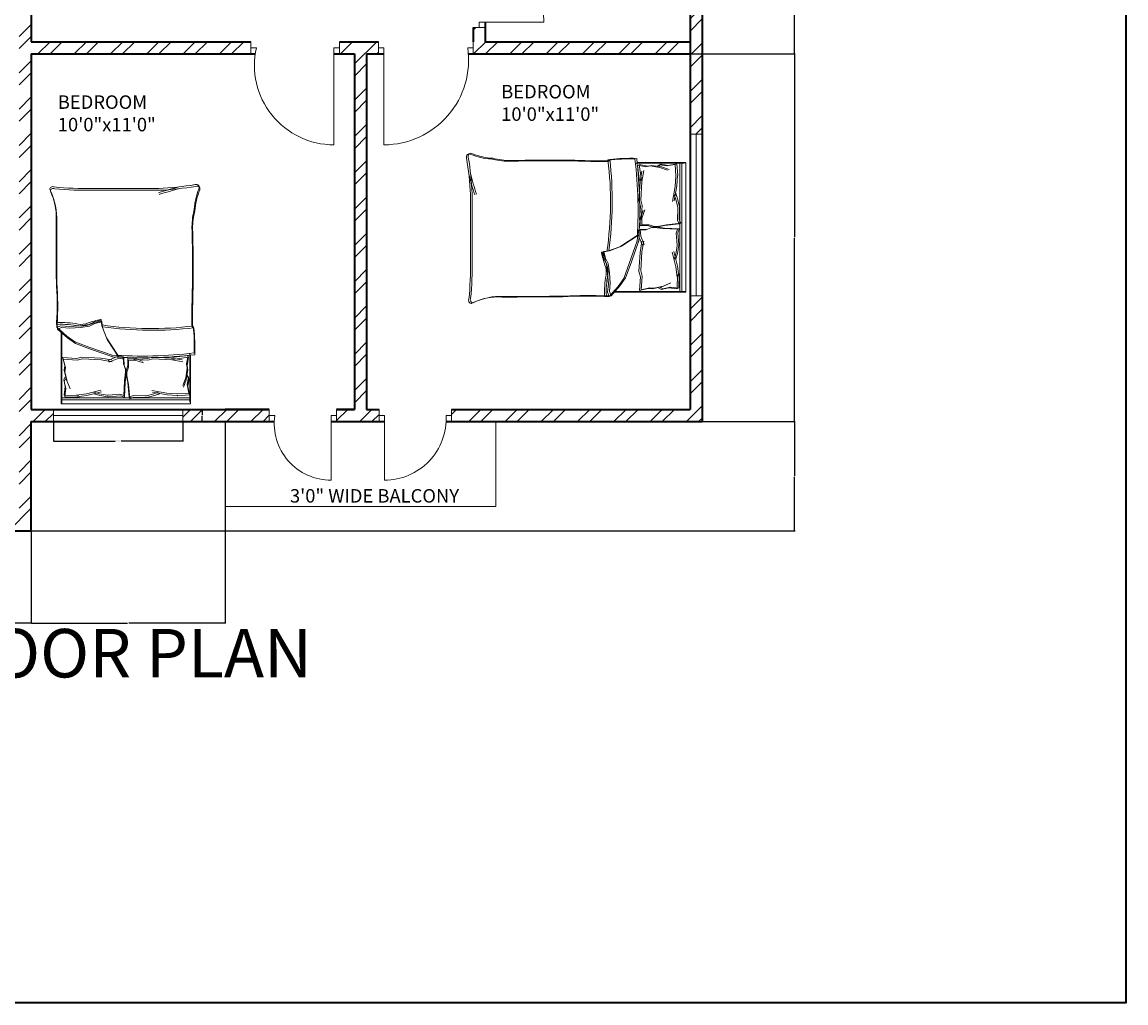
# Model space of a CAD drawing. Units: inches. Extents: x 2165 to 3042, y 1626 to 2968.
# Tile 6 of 11: x 2633 to 3042, y 1626 to 1990. Entities that reach past the tile are written whole.
import ezdxf

# ---------------------------------------------------------------- set-up
doc = ezdxf.new("R2010")
doc.units = ezdxf.units.IN
for name, color, linetype, lineweight in [('A-ANNO-DIMS', 2, 'Continuous', 18), ('A-ANNO-TEXT', 7, 'Continuous', 25), ('A-AREA-IDEN', 7, 'Continuous', 18), ('A-DOOR', 3, 'Continuous', 18), ('A-FLOR-BALC', 7, 'Continuous', 18), ('A-FURN', 8, 'Continuous', 13), ('A-GLAZ', 4, 'Continuous', 18), ('A-WALL', 7, 'Continuous', 35), ('A-WALL-PATT', 252, 'Continuous', 13)]:
    doc.layers.add(name, color=color, linetype=linetype, lineweight=lineweight)
doc.styles.get("Standard").update_dxf_attribs({"font": 'arial.ttf'})
doc.dimstyles.get("Standard").update_dxf_attribs({"dimtxt": 0.18, "dimasz": 0.18, "dimexe": 0.18, "dimexo": 0.0625, "dimgap": 0.09, "dimtad": 0, "dimtih": 1, "dimtoh": 1, "dimdec": 4, "dimzin": 0, "dimdsep": 46, "dimtxsty": 'Standard', "dimcen": 0.09, "dimadec": 0, "dimazin": 0, "dimtfac": 1, "dimtdec": 4, "dimtofl": 0, "dimtmove": 0, "dimatfit": 3, "dimfxl": 1, "dimtolj": 1, "dimtzin": 0, "dimarcsym": 0})

# ---------------------------------------------------------------- blocks, each defined once
blk = doc.blocks.new('BED-DOUBLE')
for p, q in [((0, 51.27), (0, 51.49)), ((0, 51.49), (0.64, 51.49)), ((0, 51.27), (26.61, 51.27)), ((0, 51.27), (26.61, 51.27)), ((0, 51.27), (0, 3.48)), ((0.64, 51.49), (27.25, 51.49)), ((0.64, 51.49), (27.25, 51.49)), ((1.53, 3.48), (1.53, 51.27)), ((1.53, 3.47), (1.53, 51.27)), ((2.17, 3.7), (2.17, 51.49)), ((2.17, 3.7), (2.17, 51.49)), ((2.56, 50.11), (2.46, 44.71)), ((2.56, 50.11), (2.46, 44.71)), ((2.56, 50.11), (5.77, 49.73)), ((2.56, 50.11), (5.77, 49.73)), ((3.2, 50.34), (3.1, 44.94)), ((3.2, 50.34), (3.1, 44.94)), ((3.2, 50.34), (6.41, 49.96)), ((3.2, 50.34), (6.41, 49.96)), ((8.26, 49.31), (5.58, 48.13)), ((8.26, 49.31), (5.58, 48.13)), ((5.77, 49.73), (8.34, 50.33)), ((5.77, 49.73), (8.34, 50.33)), ((8.9, 49.54), (6.22, 48.36)), ((8.9, 49.54), (6.22, 48.36)), ((6.41, 49.96), (8.98, 50.56)), ((6.41, 49.96), (8.98, 50.56)), ((11.83, 50.11), (8.26, 49.31)), ((11.83, 50.11), (8.26, 49.31)), ((8.34, 50.33), (9.38, 49.81)), ((8.34, 50.33), (9.38, 49.81)), ((12.47, 50.34), (8.9, 49.54)), ((12.47, 50.34), (8.9, 49.54)), ((8.98, 50.56), (10.02, 50.04)), ((8.98, 50.56), (10.02, 50.04)), ((13.43, 49.92), (11.83, 50.11)), ((13.43, 49.92), (11.83, 50.11)), ((14.07, 50.15), (12.47, 50.34)), ((14.07, 50.15), (12.47, 50.34)), ((16.57, 50.7), (13.43, 49.92)), ((16.57, 50.7), (13.43, 49.92)), ((17.21, 50.93), (14.07, 50.15)), ((17.21, 50.93), (14.07, 50.15)), ((16.17, 45.57), (16.57, 50.7)), ((16.17, 45.57), (16.57, 50.7)), ((16.81, 45.79), (17.21, 50.93)), ((16.81, 45.79), (17.21, 50.93)), ((24.5, 49.16), (22.33, 46.22)), ((24.5, 49.16), (22.33, 46.22)), ((25.14, 49.39), (22.97, 46.45)), ((25.14, 49.39), (22.97, 46.45)), ((27.75, 52.87), (24.5, 49.16)), ((27.75, 52.87), (24.5, 49.16)), ((28.39, 53.1), (25.14, 49.39)), ((28.39, 53.1), (25.14, 49.39)), ((29.49, 52.95), (27.75, 52.87, 3.87)), ((29.49, 52.95), (27.75, 52.87, 3.87)), ((28.37, 51.33), (27.75, 52.87)), ((28.37, 51.33), (27.75, 52.87)), ((28.06, 48.23), (28.37, 51.33)), ((28.06, 48.23), (28.37, 51.33)), ((30.13, 53.18), (28.39, 53.1, 3.87)), ((30.13, 53.18), (28.39, 53.1, 3.87)), ((29, 51.56), (28.39, 53.1)), ((29, 51.56), (28.39, 53.1)), ((28.7, 48.46), (29, 51.56)), ((28.7, 48.46), (29, 51.56)), ((2.46, 44.71), (2.54, 45.71)), ((2.46, 44.71), (2.54, 45.71)), ((2.54, 45.71), (3.07, 41.91)), ((2.54, 45.71), (3.07, 41.91)), ((3.1, 44.94), (3.18, 45.94)), ((3.1, 44.94), (3.18, 45.94)), ((3.18, 45.94), (3.71, 42.14)), ((3.18, 45.94), (3.71, 42.14)), ((16.73, 43.61), (16.17, 45.57)), ((16.73, 43.61), (16.17, 45.57)), ((17.37, 43.83), (16.81, 45.79)), ((17.37, 43.83), (16.81, 45.79)), ((22.33, 46.22), (20.32, 40.64)), ((22.33, 46.22), (20.32, 40.64)), ((22.97, 46.45), (20.96, 40.87)), ((22.97, 46.45), (20.96, 40.87)), ((28.37, 44.36), (28.06, 48.23)), ((28.37, 44.36), (28.06, 48.23)), ((29, 44.59), (28.7, 48.46)), ((29, 44.59), (28.7, 48.46)), ((3.07, 41.91), (4.42, 36.5)), ((3.07, 41.91), (4.42, 36.49)), ((3.71, 42.14), (5.06, 36.72)), ((3.71, 42.14), (5.06, 36.72)), ((16.3, 36.6), (16.73, 43.61)), ((16.3, 36.6), (16.73, 43.61)), ((16.93, 36.82), (17.37, 43.83)), ((16.93, 36.82), (17.37, 43.83)), ((28.83, 40.95), (28.37, 44.36)), ((28.83, 40.95), (28.37, 44.36)), ((29.47, 41.18), (29, 44.59)), ((29.47, 41.18), (29, 44.59)), ((30.4, 39.17), (29.47, 41.18)), ((30.4, 39.17), (29.47, 41.18)), ((3.08, 37.14), (2.54, 34.2)), ((3.08, 37.13), (2.54, 34.2)), ((3.67, 39.2), (3.08, 37.14)), ((3.67, 39.2), (3.08, 37.13)), ((3.72, 37.36), (3.18, 34.43)), ((3.72, 37.36), (3.18, 34.43)), ((4.31, 39.43), (3.72, 37.36)), ((4.31, 39.43), (3.72, 37.36)), ((20.32, 40.64), (17.38, 32.31)), ((20.32, 40.64), (17.38, 32.31)), ((20.96, 40.87), (18.02, 32.53)), ((20.96, 40.87), (18.02, 32.53)), ((29.76, 38.94), (28.83, 40.95)), ((29.76, 38.94), (28.83, 40.95)), ((30.38, 36.46), (29.76, 38.94)), ((30.38, 36.46), (29.76, 38.94)), ((31.02, 36.69), (30.4, 39.17)), ((31.02, 36.69), (30.4, 39.17)), ((79.25, 15.06), (79.25, 39.68)), ((79.25, 15.06), (79.25, 39.68)), ((79.88, 15.29), (79.88, 39.91)), ((79.88, 15.29), (79.88, 39.91)), ((2.54, 34.2), (2.56, 33.88)), ((2.54, 34.2), (2.56, 33.88)), ((2.56, 33.88), (2.98, 29.46)), ((2.56, 33.88), (2.98, 29.46)), ((3.18, 34.43), (3.2, 34.11)), ((3.18, 34.43), (3.2, 34.11)), ((3.2, 34.11), (3.62, 29.68)), ((3.2, 34.11), (3.62, 29.68)), ((16.74, 30.75), (15.46, 33.82)), ((16.74, 30.75), (15.46, 33.82)), ((15.63, 32.56), (16.3, 36.6)), ((15.63, 32.56), (16.3, 36.6)), ((17.38, 30.98), (16.09, 34.05)), ((17.38, 30.98), (16.09, 34.05)), ((16.27, 32.79), (16.93, 36.82)), ((16.27, 32.79), (16.93, 36.82)), ((17.38, 30.26), (23.88, 34.45)), ((17.38, 30.26), (23.88, 34.45)), ((18.02, 30.49), (24.52, 34.68)), ((18.02, 30.49), (24.52, 34.68)), ((23.88, 34.45), (28.37, 36.15)), ((23.88, 34.45), (28.37, 36.15)), ((24.52, 34.68), (29, 36.38)), ((24.52, 34.68), (29, 36.38)), ((28.37, 36.15), (30.38, 36.46)), ((28.37, 36.15), (30.38, 36.46)), ((29, 36.38), (31.02, 36.69)), ((29, 36.38), (31.02, 36.69)), ((2.98, 29.46), (2.49, 27.98)), ((2.98, 29.46), (2.49, 27.98)), ((3.62, 29.68), (3.13, 28.21)), ((3.62, 29.68), (3.13, 28.21)), ((16.89, 28.3), (16.74, 30.75)), ((16.89, 28.3), (16.74, 30.75)), ((17.53, 28.53), (17.38, 30.98)), ((17.53, 28.53), (17.38, 30.98)), ((1.87, 25.98), (7.22, 26.56)), ((1.87, 25.98), (7.22, 26.56)), ((2.45, 24.54), (1.87, 25.98)), ((2.45, 24.54), (1.87, 25.98)), ((2.49, 27.98), (7.87, 27.73)), ((2.49, 27.98), (7.87, 27.73)), ((2.51, 26.21), (7.86, 26.79)), ((2.51, 26.21), (7.86, 26.79)), ((3.09, 24.77), (2.51, 26.21)), ((3.09, 24.77), (2.51, 26.21)), ((2.94, 20.32), (3.09, 24.77)), ((2.94, 20.32), (3.09, 24.77)), ((3.13, 28.21), (8.51, 27.96)), ((3.13, 28.21), (8.51, 27.96)), ((7.22, 26.56), (10.4, 27.14)), ((7.22, 26.56), (10.4, 27.14)), ((7.86, 26.79), (11.04, 27.37)), ((7.86, 26.79), (11.04, 27.37)), ((7.87, 27.73), (11.08, 27.35)), ((7.87, 27.73), (11.08, 27.35)), ((8.51, 27.96), (11.72, 27.58)), ((8.51, 27.96), (11.72, 27.58)), ((10.4, 27.14), (11.7, 27.14)), ((10.4, 27.14), (11.7, 27.14)), ((11.04, 27.37), (12.34, 27.37)), ((11.04, 27.37), (12.34, 27.37)), ((11.08, 27.35), (12.38, 27.44)), ((11.08, 27.35), (12.38, 27.44)), ((11.7, 27.14), (13.58, 26.56)), ((11.7, 27.14), (13.58, 26.56)), ((11.72, 27.58), (13.02, 27.66)), ((11.72, 27.58), (13.02, 27.66)), ((12.34, 27.37), (14.22, 26.79)), ((12.34, 27.37), (14.22, 26.79)), ((12.38, 27.44), (14.22, 28.13)), ((12.38, 27.44), (14.22, 28.13)), ((13.02, 27.66), (14.86, 28.36)), ((13.02, 27.66), (14.86, 28.36)), ((13.58, 26.56), (16.26, 26.56)), ((13.58, 26.56), (16.26, 26.56)), ((14.22, 28.13), (16.89, 28.3)), ((14.22, 28.13), (16.89, 28.3)), ((14.22, 26.79), (16.9, 26.79)), ((14.22, 26.79), (16.9, 26.79)), ((14.86, 28.36), (17.53, 28.53)), ((14.86, 28.36), (17.53, 28.53)), ((16.26, 26.56), (16.26, 24.1)), ((16.26, 26.56), (16.26, 24.1)), ((16.81, 19.61), (17.21, 24.74)), ((16.81, 19.61), (17.21, 24.74)), ((16.9, 26.79), (16.9, 24.33)), ((16.9, 26.79), (16.9, 24.33)), ((2.3, 20.09), (2.45, 24.54)), ((2.3, 20.09), (2.45, 24.54)), ((16.26, 24.1), (15.17, 20.96)), ((16.26, 24.1), (15.17, 20.96)), ((16.9, 24.33), (15.81, 21.19)), ((16.9, 24.33), (15.81, 21.19)), ((16.17, 19.38), (16.57, 24.52)), ((16.17, 19.38), (16.57, 24.52)), ((2.3, 19.77), (2.3, 20.09)), ((2.3, 19.77), (2.3, 20.09)), ((3.03, 16.88), (2.3, 19.77)), ((3.03, 16.88), (2.3, 19.77)), ((2.94, 20), (2.94, 20.32)), ((2.94, 20), (2.94, 20.32)), ((3.67, 17.11), (2.94, 20)), ((3.67, 17.11), (2.94, 20)), ((3.75, 14.85), (3.03, 16.88)), ((3.75, 14.85), (3.03, 16.88)), ((3.32, 12.11), (4.33, 17.6)), ((3.32, 12.11), (4.33, 17.6)), ((4.39, 15.08), (3.67, 17.11)), ((4.39, 15.08), (3.67, 17.11)), ((3.96, 12.34), (4.97, 17.83)), ((3.96, 12.34), (4.97, 17.83)), ((16.73, 17.42), (16.17, 19.38)), ((16.73, 17.42), (16.17, 19.38)), ((16.3, 10.41), (16.73, 17.42)), ((16.3, 10.41), (16.73, 17.42)), ((17.37, 17.65), (16.81, 19.61)), ((17.37, 17.65), (16.81, 19.61)), ((16.93, 10.64), (17.37, 17.65)), ((16.93, 10.64), (17.37, 17.65)), ((3.67, 8.51), (3.96, 12.34)), ((3.67, 8.51), (3.96, 12.34)), ((3.01, 8.18), (3.03, 8.28)), ((3.01, 8.18), (3.03, 8.28)), ((3.03, 8.28), (3.32, 12.11)), ((3.03, 8.28), (3.32, 12.11)), ((3.65, 8.41), (3.67, 8.51)), ((3.65, 8.41), (3.67, 8.51)), ((3.98, 4.13), (3.65, 8.41)), ((3.98, 4.13), (3.65, 8.41)), ((15.63, 6.38), (16.3, 10.41)), ((15.63, 6.38), (16.3, 10.41)), ((16.27, 6.61), (16.93, 10.64)), ((16.27, 6.61), (16.93, 10.64)), ((16.3, 10.41), (16.62, 9.28)), ((16.3, 10.41), (16.62, 9.28)), ((16.62, 9.28), (17.34, 4.18)), ((16.62, 9.28), (17.34, 4.18)), ((16.93, 10.64), (17.26, 9.51)), ((16.93, 10.64), (17.26, 9.51)), ((17.26, 9.51), (17.98, 4.41)), ((17.26, 9.51), (17.98, 4.41)), ((3.34, 3.9), (3.01, 8.18)), ((3.34, 3.9), (3.01, 8.18)), ((3.32, 3.89), (6.5, 4.47)), ((3.32, 3.89), (6.5, 4.47)), ((3.96, 4.12), (7.14, 4.7)), ((3.96, 4.12), (7.14, 4.7)), ((8.96, 5.05), (6.21, 6.06)), ((8.96, 5.05), (6.21, 6.06)), ((6.5, 4.47), (9.1, 4.04)), ((6.5, 4.47), (9.1, 4.04)), ((9.59, 5.28), (6.85, 6.29)), ((9.59, 5.28), (6.85, 6.29)), ((7.14, 4.7), (9.74, 4.27)), ((7.14, 4.7), (9.74, 4.27)), ((12.57, 4.47), (8.96, 5.05)), ((12.57, 4.47), (8.96, 5.05)), ((9.1, 4.04), (10.11, 4.62)), ((9.1, 4.04), (10.11, 4.62)), ((13.21, 4.7), (9.59, 5.28)), ((13.21, 4.7), (9.59, 5.28)), ((9.74, 4.27), (10.75, 4.85)), ((9.74, 4.27), (10.75, 4.85)), ((14.16, 4.76), (12.57, 4.47)), ((14.16, 4.76), (12.57, 4.47)), ((14.8, 4.99), (13.21, 4.7)), ((14.8, 4.99), (13.21, 4.7)), ((17.34, 4.18), (14.16, 4.76)), ((17.34, 4.18), (14.16, 4.76)), ((17.98, 4.41), (14.8, 4.99)), ((17.98, 4.41), (14.8, 4.99)), ((18.11, 3.48), (0, 3.48)), ((18.11, 3.47), (0, 3.47)), ((18.75, 3.7), (0.64, 3.7)), ((18.75, 3.7), (0.64, 3.7))]:
    blk.add_line(p, q)
for centre, radius, start, end in [((36.95, 182.49), 129.5, 266.9791, 273.8365), ((36.95, 182.49), 129.5, 266.9791, 273.8365), ((68.46, -4508.52), 4561.86, 90.00217, 90.28689), ((68.46, -4508.52), 4561.86, 90.00217, 90.28689), ((68.67, 76.16), 23.07, 267.4714, 296.4681), ((68.67, 76.16), 23.07, 267.4714, 296.4681), ((69.31, 76.39), 23.07, 267.4714, 296.4681), ((69.31, 76.39), 23.07, 267.4714, 296.4681), ((78.87, 54.41), 1.1, 332.6588, 86.02), ((78.87, 54.41), 1.1, 332.6588, 86.02), ((212.28, 41.15), 133.04, 174.4998, 180.6351), ((212.28, 41.15), 133.04, 174.4998, 180.6351), ((79.51, 54.64), 1.1, 332.6588, 86.02), ((79.51, 54.64), 1.1, 332.6588, 86.02), ((212.92, 41.38), 133.04, 174.4998, 180.6351), ((212.92, 41.38), 133.04, 174.4998, 180.6351), ((-6.66, 51.33), 36.18, 349.8763, 2.5657), ((-6.66, 51.33), 36.18, 349.8763, 2.5657), ((36.32, 182.27), 129.5, 266.9791, 273.8365), ((36.32, 182.27), 129.5, 266.9791, 273.8365), ((-6.02, 51.56), 36.18, 349.8763, 2.5657), ((-6.02, 51.56), 36.18, 349.8763, 2.5657), ((67.82, -4508.74), 4561.86, 90.00217, 90.28689), ((67.82, -4508.74), 4561.86, 90.00217, 90.28689), ((35.71, 43.97), 6.22, 168.6608, 203.7384), ((35.71, 43.97), 6.22, 168.6608, 203.7384), ((35.07, 43.74), 6.22, 168.6608, 203.7384), ((35.07, 43.74), 6.22, 168.6608, 203.7384), ((1.48, 31.15), 29.65, 10.6617, 19.8806), ((1.48, 31.15), 29.65, 10.6617, 19.8806), ((2.12, 31.38), 29.65, 10.6617, 19.8806), ((2.12, 31.38), 29.65, 10.6617, 19.8806), ((31.08, 36.86), 0.185, 250.2464, 1.1377), ((31.08, 36.86), 0.185, 250.2464, 1.1377), ((182.69, 21.59), 164.97, 176.0865, 186.7821), ((182.69, 21.59), 164.97, 176.0865, 186.7821), ((156.32, 17.76), 129.02, 171.7845, 186.9006), ((156.32, 17.76), 129.02, 171.7845, 186.9006), ((156.96, 17.98), 129.02, 171.7845, 186.9006), ((156.96, 17.98), 129.02, 171.7845, 186.9006), ((30.44, 36.64), 0.185, 250.2464, 1.1377), ((30.44, 36.64), 0.185, 250.2464, 1.1377), ((182.05, 21.36), 164.97, 176.0865, 186.7821), ((182.05, 21.36), 164.97, 176.0865, 186.7821), ((-23.71, -17.22), 106.46, 13.3832, 17.7053), ((-23.71, -17.22), 106.46, 13.3832, 17.7053), ((-23.07, -16.99), 106.46, 13.3832, 17.7053), ((-23.07, -16.99), 106.46, 13.3832, 17.7053), ((200.84, 21.43), 121.76, 182.9958, 189.4091), ((200.84, 21.43), 121.76, 182.9958, 189.4091), ((201.48, 21.66), 121.76, 182.9958, 189.4091), ((201.48, 21.65), 121.76, 182.9958, 189.4091), ((20.1, 85.16), 83.31, 268.7218, 275.604), ((20.1, 85.16), 83.31, 268.7218, 275.604), ((20.74, 85.39), 83.31, 268.7218, 275.604), ((20.74, 85.39), 83.31, 268.7218, 275.604), ((31.17, -167.31), 170.11, 88.4762, 91.0082), ((31.17, -167.31), 170.11, 88.4762, 91.0082), ((31.81, -167.08), 170.11, 88.4762, 91.0082), ((31.81, -167.08), 170.11, 88.4762, 91.0082), ((50.61, 484.82), 482.31, 268.2277, 271.7185), ((50.61, 484.82), 482.31, 268.2277, 271.7185), ((51.25, 485.05), 482.31, 268.2277, 271.7185), ((51.25, 485.05), 482.31, 268.2277, 271.7185), ((64.52, -26.9), 29.63, 76.0648, 88.9113), ((64.52, -26.9), 29.63, 76.0648, 88.9113), ((65.15, -26.67), 29.63, 76.0648, 88.9113), ((65.15, -26.67), 29.63, 76.0648, 88.9113), ((70.28, -21.66), 23.56, 67.9751, 86.652), ((70.28, -21.66), 23.56, 67.9751, 86.652), ((70.92, -21.43), 23.56, 67.9751, 86.652), ((70.92, -21.43), 23.56, 67.9751, 86.652), ((79.72, 1.09), 1.09, 236.1736, 23.4781), ((79.72, 1.09), 1.09, 236.1736, 23.4781), ((80.36, 1.32), 1.09, 236.1736, 23.4781), ((80.36, 1.32), 1.09, 236.1736, 23.4781)]:
    blk.add_arc(centre, radius, start, end)
blk = doc.blocks.new('BALCONY-RAIL-PLAN')
for p, q in [((0, 31.5), (0, 0)), ((100.5, 31.5), (100.5, 0)), ((100.5, 0), (0, 0))]:
    blk.add_line(p, q)
blk = doc.blocks.new('WIN-60-B')
for p, q in [((0, 4.5), (0, 0)), ((60, 2.25), (60, 4.5)), ((60, 4.5), (60, 0)), ((0, 0), (0, 2.25)), ((0, 2.25), (60, 2.25))]:
    blk.add_line(p, q)
blk = doc.blocks.new('WIN-48')
for p, q in [((0, 4.5), (0, 0)), ((48, 2.25), (48, 4.5)), ((48, 4.5), (48, 0)), ((0, 0), (0, 2.25)), ((0, 2.25), (48, 2.25))]:
    blk.add_line(p, q)
blk = doc.blocks.new('*D36')
at = {"layer": 'A-ANNO-DIMS', "color": 0, "lineweight": -2, "transparency": 16777216}
for p, q in [((2644.34, 1842.02), (2644.34, 1834.7)), ((2692.34, 1842.02), (2692.34, 1834.7)), ((2644.52, 1834.88), (2667.22, 1834.88)), ((2692.16, 1834.88), (2669.46, 1834.88))]:
    blk.add_line(p, q, dxfattribs=at)
at = {"layer": 'A-ANNO-DIMS', "color": 0, "transparency": 16777216}
for points in [[(2644.52, 1834.91), (2644.52, 1834.85), (2644.34, 1834.88)], [(2692.16, 1834.91), (2692.16, 1834.85), (2692.34, 1834.88)]]:
    blk.add_solid(points, dxfattribs=at)
at = {"layer": 'Defpoints', "color": 0, "transparency": 16777216}
for p in [(2644.34, 1842.08), (2692.34, 1842.08), (2692.34, 1834.88)]:
    blk.add_point(p, dxfattribs=at)
at = {"layer": 'A-ANNO-DIMS', "color": 0, "transparency": 16777216, "insert": (2668.34, 1834.88), "char_height": 0.18, "attachment_point": 5}
blk.add_mtext('\\A1;WINDOW 48 TYP.', dxfattribs=at)
blk = doc.blocks.new('*D37')
at = {"layer": 'A-ANNO-DIMS', "color": 0, "lineweight": -2, "transparency": 16777216}
for p, q in [((2692.4, 1846.58), (2699.72, 1846.58)), ((2699.54, 1846.4), (2699.54, 1844.51)), ((2699.54, 1842.26), (2699.54, 1844.15)), ((2692.4, 1842.08), (2699.72, 1842.08))]:
    blk.add_line(p, q, dxfattribs=at)
at = {"layer": 'A-ANNO-DIMS', "color": 0, "transparency": 16777216}
for points in [[(2699.51, 1846.4), (2699.57, 1846.4), (2699.54, 1846.58)], [(2699.51, 1842.26), (2699.57, 1842.26), (2699.54, 1842.08)]]:
    blk.add_solid(points, dxfattribs=at)
at = {"layer": 'Defpoints', "color": 0, "transparency": 16777216}
for p in [(2692.34, 1846.58), (2699.54, 1846.58), (2692.34, 1842.08)]:
    blk.add_point(p, dxfattribs=at)
at = {"layer": 'A-ANNO-DIMS', "color": 0, "transparency": 16777216, "insert": (2699.54, 1844.33), "char_height": 0.18, "attachment_point": 5}
blk.add_mtext('\\A1;5 TYP.', dxfattribs=at)
blk = doc.blocks.new('*D54')
at = {"layer": 'A-ANNO-DIMS', "color": 0, "lineweight": -2, "transparency": 16777216}
for p, q in [((2535.6, 1801.52), (2535.6, 1767.1)), ((2636.1, 1801.52), (2636.1, 1767.1)), ((2535.78, 1767.28), (2585.47, 1767.28)), ((2635.92, 1767.28), (2586.24, 1767.28))]:
    blk.add_line(p, q, dxfattribs=at)
at = {"layer": 'A-ANNO-DIMS', "color": 0, "transparency": 16777216}
for points in [[(2535.78, 1767.31), (2535.78, 1767.25), (2535.6, 1767.28)], [(2635.92, 1767.31), (2635.92, 1767.25), (2636.1, 1767.28)]]:
    blk.add_solid(points, dxfattribs=at)
at = {"layer": 'Defpoints', "color": 0, "transparency": 16777216}
for p in [(2535.6, 1801.58), (2636.1, 1801.58), (2636.1, 1767.28)]:
    blk.add_point(p, dxfattribs=at)
at = {"layer": 'A-ANNO-DIMS', "color": 0, "transparency": 16777216, "insert": (2585.85, 1767.28), "char_height": 0.18, "attachment_point": 5}
blk.add_mtext('\\A1;100.5', dxfattribs=at)
blk = doc.blocks.new('*D55')
at = {"layer": 'A-ANNO-DIMS', "color": 0, "lineweight": -2, "transparency": 16777216}
for p, q in [((2636.1, 1842.02), (2636.1, 1767.1)), ((2708.1, 1842.02), (2708.1, 1767.1)), ((2636.28, 1767.28), (2671.89, 1767.28)), ((2707.92, 1767.28), (2672.32, 1767.28))]:
    blk.add_line(p, q, dxfattribs=at)
at = {"layer": 'A-ANNO-DIMS', "color": 0, "transparency": 16777216}
for points in [[(2636.28, 1767.31), (2636.28, 1767.25), (2636.1, 1767.28)], [(2707.92, 1767.31), (2707.92, 1767.25), (2708.1, 1767.28)]]:
    blk.add_solid(points, dxfattribs=at)
at = {"layer": 'Defpoints', "color": 0, "transparency": 16777216}
for p in [(2636.1, 1842.08), (2708.1, 1842.08), (2708.1, 1767.28)]:
    blk.add_point(p, dxfattribs=at)
at = {"layer": 'A-ANNO-DIMS', "color": 0, "transparency": 16777216, "insert": (2672.1, 1767.28), "char_height": 0.18, "attachment_point": 5}
blk.add_mtext('\\A1;72', dxfattribs=at)
blk = doc.blocks.new('*D56')
at = {"layer": 'A-ANNO-DIMS', "color": 0, "lineweight": -2, "transparency": 16777216}
for p, q in [((2885.17, 1842.08), (2919.58, 1842.08)), ((2919.4, 1841.9), (2919.4, 1822.01)), ((2919.4, 1801.76), (2919.4, 1821.65)), ((2636.17, 1801.58), (2919.58, 1801.58))]:
    blk.add_line(p, q, dxfattribs=at)
at = {"layer": 'A-ANNO-DIMS', "color": 0, "transparency": 16777216}
for points in [[(2919.37, 1841.9), (2919.43, 1841.9), (2919.4, 1842.08)], [(2919.37, 1801.76), (2919.43, 1801.76), (2919.4, 1801.58)]]:
    blk.add_solid(points, dxfattribs=at)
at = {"layer": 'Defpoints', "color": 0, "transparency": 16777216}
for p in [(2885.1, 1842.08), (2919.4, 1842.08), (2636.1, 1801.58)]:
    blk.add_point(p, dxfattribs=at)
at = {"layer": 'A-ANNO-DIMS', "color": 0, "transparency": 16777216, "insert": (2919.4, 1821.83), "char_height": 0.18, "attachment_point": 5}
blk.add_mtext('\\A1;40.5', dxfattribs=at)
blk = doc.blocks.new('*D57')
at = {"layer": 'A-ANNO-DIMS', "color": 0, "lineweight": -2, "transparency": 16777216}
for p, q in [((2880.67, 1978.58), (2919.58, 1978.58)), ((2919.4, 1978.4), (2919.4, 1910.51)), ((2919.4, 1842.26), (2919.4, 1910.15)), ((2885.17, 1842.08), (2919.58, 1842.08))]:
    blk.add_line(p, q, dxfattribs=at)
at = {"layer": 'A-ANNO-DIMS', "color": 0, "transparency": 16777216}
for points in [[(2919.37, 1978.4), (2919.43, 1978.4), (2919.4, 1978.58)], [(2919.37, 1842.26), (2919.43, 1842.26), (2919.4, 1842.08)]]:
    blk.add_solid(points, dxfattribs=at)
at = {"layer": 'Defpoints', "color": 0, "transparency": 16777216}
for p in [(2880.6, 1978.58), (2919.4, 1978.58), (2885.1, 1842.08)]:
    blk.add_point(p, dxfattribs=at)
at = {"layer": 'A-ANNO-DIMS', "color": 0, "transparency": 16777216, "insert": (2919.4, 1910.33), "char_height": 0.18, "attachment_point": 5}
blk.add_mtext('\\A1;136.5', dxfattribs=at)
blk = doc.blocks.new('*D58')
at = {"layer": 'A-ANNO-DIMS', "color": 0, "lineweight": -2, "transparency": 16777216}
for p, q in [((2885.17, 2075.58), (2919.58, 2075.58)), ((2919.4, 2075.4), (2919.4, 2027.26)), ((2919.4, 1978.76), (2919.4, 2026.9)), ((2880.67, 1978.58), (2919.58, 1978.58))]:
    blk.add_line(p, q, dxfattribs=at)
at = {"layer": 'A-ANNO-DIMS', "color": 0, "transparency": 16777216}
for points in [[(2919.37, 2075.4), (2919.43, 2075.4), (2919.4, 2075.58)], [(2919.37, 1978.76), (2919.43, 1978.76), (2919.4, 1978.58)]]:
    blk.add_solid(points, dxfattribs=at)
at = {"layer": 'Defpoints', "color": 0, "transparency": 16777216}
for p in [(2885.1, 2075.58), (2919.4, 2075.58), (2880.6, 1978.58)]:
    blk.add_point(p, dxfattribs=at)
at = {"layer": 'A-ANNO-DIMS', "color": 0, "transparency": 16777216, "insert": (2919.4, 2027.08), "char_height": 0.18, "attachment_point": 5}
blk.add_mtext('\\A1;97', dxfattribs=at)

msp = doc.modelspace()

# ---------------------------------------------------------------- hatches: boundary and pattern name
at = {"layer": 'A-WALL-PATT'}
h = msp.add_hatch(dxfattribs=at)
h.set_pattern_fill('ANSI32', color=256)
h.paths.add_polyline_path([(2406.4931, 2332.0783), (2286.6045, 2332.0783), (2286.6045, 2310.967), (2288.8545, 2310.967), (2291.1045, 2310.967), (2291.1045, 2327.5783), (2406.4931, 2327.5783), (2406.4931, 2329.8283)])
h.paths.add_polyline_path([(2439.6045, 2327.5783), (2444.9584, 2327.5783), (2444.9584, 2332.0783), (2430.2901, 2332.0783), (2430.2901, 2329.8283), (2430.2901, 2327.5783), (2435.1045, 2327.5783), (2435.1045, 2219.5783), (2431.0902, 2219.5783), (2431.0902, 2215.0783), (2435.1045, 2215.0783), (2444.1108, 2215.0783), (2444.1108, 2217.3283), (2444.1108, 2219.5783), (2439.6045, 2219.5783)])
h.paths.add_polyline_path([(2497.5418, 2329.8283), (2497.5418, 2332.0783), (2470.1978, 2332.0783), (2470.1978, 2327.5783), (2497.5418, 2327.5783)])
h.paths.add_polyline_path([(2617.9543, 2332.0783), (2557.5418, 2332.0783), (2557.5418, 2327.5783), (2583.6045, 2327.5783), (2583.6045, 2219.5783), (2474.0523, 2219.5783), (2474.0523, 2215.0783), (2583.6045, 2215.0783), (2583.6045, 2107.0783), (2579.3609, 2107.0783), (2579.3609, 2102.5783), (2588.1045, 2102.5783), (2593.5283, 2102.5783), (2593.5283, 2104.8283), (2593.5283, 2107.0783), (2588.1045, 2107.0783), (2588.1045, 2215.0783), (2691.2325, 2215.0783), (2691.2325, 2217.3283), (2691.2325, 2219.5783), (2588.1045, 2219.5783), (2588.1045, 2327.5783), (2617.9543, 2327.5783)])
h.paths.add_polyline_path([(2702.4444, 2329.8283), (2702.4444, 2332.0783), (2677.9543, 2332.0783), (2677.9543, 2327.5783), (2702.4444, 2327.5783)])
h.paths.add_polyline_path([(2736.6045, 2327.5783), (2742.5161, 2327.5783), (2742.5161, 2329.8283), (2742.5161, 2332.0783), (2727.7639, 2332.0783), (2727.7639, 2329.8283), (2727.7639, 2327.5783), (2732.1045, 2327.5783), (2732.1045, 2219.5783), (2726.4404, 2219.5783), (2726.4404, 2215.0783), (2732.1045, 2215.0783), (2742.7291, 2215.0783), (2742.7291, 2217.3283), (2742.7291, 2219.5783), (2736.6045, 2219.5783)])
h.paths.add_polyline_path([(2885.1045, 2332.0783), (2768.4887, 2332.0783), (2768.4887, 2327.5783), (2784.6045, 2327.5783), (2880.6045, 2327.5783), (2880.6045, 2310.967), (2885.1045, 2310.967)])
h.paths.add_polyline_path([(2885.1045, 2250.967), (2880.6045, 2250.967), (2880.6045, 2219.5783), (2776.5755, 2219.5783), (2776.5755, 2215.0783), (2788.1045, 2215.0783), (2788.1045, 2209.8634), (2790.3545, 2209.8634), (2792.6045, 2209.8634), (2792.6045, 2215.0783), (2880.6045, 2215.0783), (2880.6045, 2139.0783), (2871.2037, 2139.0783), (2871.2037, 2134.5783), (2885.1045, 2134.5783)])
h.paths.add_polyline_path([(2545.013, 2107.0783), (2474.0523, 2107.0783), (2291.1045, 2107.0783), (2291.1045, 2102.5783), (2535.6045, 2102.5783), (2535.6045, 2096.8046), (2537.8545, 2096.8046), (2540.1045, 2096.8046), (2540.1045, 2102.5783), (2545.013, 2102.5783), (2545.013, 2104.8283)])
h.paths.add_polyline_path([(2397.7297, 2217.3283), (2397.7297, 2219.5783), (2291.1045, 2219.5783), (2291.1045, 2250.967), (2286.6045, 2250.967), (2286.6045, 2206.1346), (2288.8545, 2206.1346), (2291.1045, 2206.1346), (2291.1045, 2215.0783), (2367.1045, 2215.0783), (2367.1045, 2212.2868), (2371.6045, 2212.2868), (2371.6045, 2215.0783), (2397.7297, 2215.0783)])
h.paths.add_polyline_path([(2291.1045, 1978.5783), (2367.1045, 1978.5783), (2371.6045, 1978.5783), (2373.2641, 1978.5783), (2374.4883, 1978.5783), (2374.4883, 1980.8283), (2374.4883, 1983.0783), (2371.6045, 1983.0783), (2371.6045, 1986.964), (2369.9051, 1986.964), (2369.3545, 1986.964), (2367.1045, 1986.964), (2367.1045, 1983.0783), (2291.1045, 1983.0783), (2291.1045, 2001.1808), (2286.6045, 2001.1808), (2286.6045, 1947.0203), (2288.8545, 1947.0203), (2291.1045, 1947.0203)])
h.paths.add_polyline_path([(2291.1045, 1887.0203), (2286.6045, 1887.0203), (2286.6045, 1842.0783), (2381.2561, 1842.0783), (2381.2561, 1844.3283), (2381.2561, 1846.5783), (2363.1045, 1846.5783), (2291.1045, 1846.5783)])
h.paths.add_polyline_path([(2415.6045, 1978.5783), (2421.1681, 1978.5783), (2421.1681, 1983.0783), (2415.6045, 1983.0783), (2406.5227, 1983.0783), (2406.5227, 1980.8283), (2406.5227, 1978.5783), (2411.1045, 1978.5783), (2411.1045, 1846.5783), (2406.7549, 1846.5783), (2406.7549, 1842.0783), (2419.2885, 1842.0783), (2419.2885, 1844.3283), (2419.2885, 1846.5783), (2415.6045, 1846.5783)])
h.paths.add_polyline_path([(2586.6045, 1982.779), (2586.6045, 1991.5911), (2582.1045, 1991.5911), (2582.1045, 1982.779), (2540.1045, 1982.779), (2540.1045, 2036.779), (2582.1045, 2036.779), (2582.1045, 2027.6051), (2586.6045, 2027.6051), (2586.6045, 2041.279), (2582.1045, 2041.279), (2540.1045, 2041.279), (2540.1045, 2063.9064), (2537.8545, 2063.9064), (2535.6045, 2063.9064), (2535.6045, 1983.0783), (2455.068, 1983.0783), (2455.068, 1978.5783), (2535.6045, 1978.5783), (2535.6045, 1846.5783), (2522.622, 1846.5783), (2522.622, 1842.0783), (2535.6045, 1842.0783), (2535.6045, 1806.0783), (2535.6045, 1801.5783), (2556.726, 1801.5783), (2556.726, 1803.8283), (2556.726, 1806.0783), (2540.1045, 1806.0783), (2540.1045, 1842.0783), (2540.1045, 1846.5783), (2540.1045, 1978.279), (2586.6045, 1978.279)])
h.paths.add_polyline_path([(2636.1045, 1978.5783), (2717.6642, 1978.5783), (2717.6642, 1980.8283), (2717.6642, 1983.0783), (2636.1045, 1983.0783), (2636.1045, 2063.9064), (2633.8545, 2063.9064), (2631.6045, 2063.9064), (2631.6045, 1846.5783), (2631.6045, 1842.0783), (2631.6045, 1806.0783), (2604.726, 1806.0783), (2604.726, 1801.5783), (2636.1045, 1801.5783), (2636.1045, 1842.0783), (2644.3411, 1842.0783), (2644.3411, 1844.3283), (2644.3411, 1846.5783), (2636.1045, 1846.5783)])
h.paths.add_polyline_path([(2760.6045, 1978.5783), (2764.9931, 1978.5783), (2764.9931, 1983.0783), (2750.4727, 1983.0783), (2750.4727, 1980.8283), (2750.4727, 1978.5783), (2756.1045, 1978.5783), (2756.1045, 1846.5783), (2749.4543, 1846.5783), (2749.4543, 1842.0783), (2765.1894, 1842.0783), (2765.1894, 1846.5783), (2760.6045, 1846.5783)])
h.paths.add_polyline_path([(2880.6045, 1983.0783), (2804.6045, 1983.0783), (2804.6045, 1988.3825), (2802.3545, 1988.3825), (2800.1045, 1988.3825), (2800.1045, 1983.0783), (2800.1045, 1978.5783), (2880.6045, 1978.5783)])
h.paths.add_polyline_path([(2885.1045, 2075.5783), (2871.2037, 2075.5783), (2871.2037, 2071.0783), (2880.6045, 2071.0783), (2880.6045, 1948.8144), (2885.1045, 1948.8144)])
h.paths.add_polyline_path([(2885.1045, 1888.8144), (2880.6045, 1888.8144), (2880.6045, 1846.5783), (2792.1167, 1846.5783), (2792.1167, 1842.0783), (2885.1045, 1842.0783)])
h.paths.add_polyline_path([(2724.4848, 1846.5783), (2708.1045, 1846.5783), (2692.3411, 1846.5783), (2692.3411, 1842.0783), (2724.4848, 1842.0783), (2724.4848, 1844.3283)])
h.paths.add_polyline_path([(2474.622, 1844.4672), (2474.622, 1846.5783), (2444.7417, 1846.5783), (2444.7417, 1842.0783), (2474.622, 1842.0783)])

# ---------------------------------------------------------------- linework, layer by layer
at = {"layer": 'A-DOOR'}
for p, q in [((2800.1045, 1988.3825), (2804.6045, 1988.3825)), ((2802.3545, 1988.3825), (2802.3545, 1990.3825)), ((2802.3545, 1990.3825), (2826.3545, 1990.3825)), ((2804.6045, 1988.3825), (2802.3545, 1988.3825)), ((2717.6642, 1983.0783), (2717.6642, 1978.5783)), ((2750.4727, 1978.5783), (2750.4727, 1983.0783)), ((2750.4727, 1983.0783), (2750.4727, 1980.8283)), ((2764.9931, 1978.5783), (2764.9931, 1983.0783)), ((2764.9931, 1983.0783), (2764.9931, 1980.8283)), ((2800.1045, 1983.0783), (2800.1045, 1978.5783)), ((2717.6642, 1978.5783), (2717.6642, 1980.8283)), ((2717.6642, 1980.8283), (2719.6642, 1980.8283)), ((2750.4727, 1980.8283), (2748.4727, 1980.8283)), ((2748.4727, 1980.8283), (2748.4727, 1944.8283)), ((2764.9931, 1980.8283), (2766.9931, 1980.8283)), ((2766.9931, 1980.8283), (2766.9931, 1944.8283)), ((2800.1045, 1980.8283), (2798.1045, 1980.8283)), ((2800.1045, 1978.5783), (2800.1045, 1980.8283)), ((2724.4848, 1846.5783), (2724.4848, 1842.0783)), ((2724.4848, 1842.0783), (2724.4848, 1844.3283)), ((2724.4848, 1844.3283), (2726.4848, 1844.3283)), ((2749.4543, 1844.3283), (2747.4543, 1844.3283)), ((2747.4543, 1844.3283), (2747.4543, 1820.3283)), ((2749.4543, 1846.5783), (2749.4543, 1842.0783)), ((2749.4543, 1842.0783), (2749.4543, 1844.3283)), ((2765.1894, 1846.5783), (2765.1894, 1842.0783)), ((2765.1894, 1844.3283), (2767.1894, 1844.3283)), ((2767.1894, 1844.3283), (2767.1894, 1820.3283)), ((2792.1167, 1844.3283), (2790.1167, 1844.3283)), ((2792.1167, 1846.5783), (2792.1167, 1842.0783)), ((2792.1167, 1842.0783), (2792.1167, 1844.3283))]:
    msp.add_line(p, q, dxfattribs=at)
for centre, radius, start, end in [((2806.4834, 1990.3825), 19.8711, 0, 102.042606), ((2748.4727, 1974.3551), 29.5268, 167.336035, 270), ((2766.9931, 1976.2716), 31.4433, 270, 8.332628), ((2747.4543, 1841.4891), 21.1608, 172.289344, 270), ((2767.1894, 1843.2796), 22.9513, 270, 2.618855)]:
    msp.add_arc(centre, radius, start, end, dxfattribs=at)
at = {"layer": 'A-WALL'}
for p, q in [((2885.1045, 2075.5783), (2885.1045, 1842.0783)), ((2880.6045, 2071.0783), (2880.6045, 1846.5783)), ((2636.1045, 2065.4985), (2636.1045, 1983.0783)), ((2800.1045, 1988.3825), (2800.1045, 1983.0783)), ((2804.6045, 1990.3825), (2804.6045, 1983.0783)), ((2636.1045, 1983.0783), (2717.6642, 1983.0783)), ((2750.4727, 1983.0783), (2764.9931, 1983.0783)), ((2804.6045, 1983.0783), (2880.6045, 1983.0783)), ((2636.1045, 1978.5783), (2719.2495, 1978.5783)), ((2636.1045, 1978.5783), (2636.1045, 1846.5783)), ((2748.4727, 1978.5783), (2756.1045, 1978.5783)), ((2756.1045, 1978.5783), (2756.1045, 1846.5783)), ((2760.6045, 1978.5783), (2760.6045, 1846.5783)), ((2760.6045, 1978.5783), (2766.9931, 1978.5783)), ((2798.3517, 1978.5783), (2880.6045, 1978.5783)), ((2636.1045, 1846.5783), (2724.4848, 1846.5783)), ((2724.4848, 1846.5783), (2708.1045, 1846.5783)), ((2756.1045, 1846.5783), (2749.4543, 1846.5783)), ((2749.4543, 1846.5783), (2756.1045, 1846.5783)), ((2760.6045, 1846.5783), (2765.1894, 1846.5783)), ((2760.6045, 1846.5783), (2765.1894, 1846.5783)), ((2792.1167, 1846.5783), (2880.6045, 1846.5783)), ((2792.1167, 1846.5783), (2808.6045, 1846.5783)), ((2636.1045, 1801.5783), (2636.1045, 1842.0783)), ((2636.1045, 1842.0783), (2726.3017, 1842.0783)), ((2747.4543, 1842.0783), (2767.1894, 1842.0783)), ((2790.1092, 1842.0783), (2885.1045, 1842.0783)), ((2535.6045, 1801.5783), (2636.1045, 1801.5783))]:
    msp.add_line(p, q, dxfattribs=at)
msp.add_lwpolyline([(2191.9961, 2967.8547), (3042.3708, 2967.8547), (3042.3708, 1626.3264), (2191.9961, 1626.3264)], close=True, dxfattribs=at)

# ---------------------------------------------------------------- block references
at = {"layer": 'A-FLOR-BALC'}
msp.add_blockref('BALCONY-RAIL-PLAN', (2708.104, 1810.578), dxfattribs=at)
at = {"layer": 'A-FURN'}
for p, rotation in [((2879.0418, 1941.6756), 180), ((2698.73, 1848.6928), 89.9999998332427)]:
    msp.add_blockref('BED-DOUBLE', p, dxfattribs=dict(at, rotation=rotation))
at = {"layer": 'A-GLAZ', "extrusion": (0, 0, -1), "zscale": -1, "rotation": 90}
msp.add_blockref('WIN-60-B', (-2880.6041, 1888.8146), dxfattribs=at)
at = {"layer": 'A-GLAZ'}
msp.add_blockref('WIN-48', (2644.341, 1842.078), dxfattribs=at)

# ---------------------------------------------------------------- texts
at = {"layer": 'A-ANNO-TEXT', "insert": (2523.1237, 1765.1301), "char_height": 18, "attachment_point": 1}
msp.add_mtext_dynamic_manual_height_columns('FIRST FLOOR PLAN', width=534.683278, gutter_width=12.5, heights=[0], dxfattribs=at)
at = {"layer": 'A-AREA-IDEN', "char_height": 5, "attachment_point": 1}
for s, width, insert in [('BEDROOM\\P10\'0"x11\'0"', 129.854383, (2810.5211, 1967.0478)), ('BEDROOM\\P10\'0"x11\'0"', 112.668669, (2645.9777, 1963.172)), ('3\'0" WIDE BALCONY', 69.420923, (2732.1316, 1817.0342))]:
    msp.add_mtext_dynamic_manual_height_columns(s, width=width, gutter_width=12.5, heights=[0], dxfattribs=dict(at, insert=insert))

# ---------------------------------------------------------------- dimensions: what is measured, and where the dimension line sits
at = {"layer": 'A-ANNO-DIMS'}
for base, p1, p2, override, picture, middle in [((2919.4045, 2075.5783), (2880.6045, 1978.5783), (2885.1045, 2075.5783), {"dimdec": 0, "dimlfac": 1, "dimrnd": 0, "dimzin": 0, "dimdsep": 46, "dimlunit": 2}, '*D58', (2919.4045, 2027.0783)), ((2919.4045, 1978.5783), (2885.1045, 1842.0783), (2880.6045, 1978.5783), {"dimdec": 1, "dimlfac": 1, "dimrnd": 0, "dimzin": 0, "dimdsep": 46, "dimlunit": 2}, '*D57', (2919.4045, 1910.3283)), ((2919.4045, 1842.0783), (2636.1045, 1801.5783), (2885.1045, 1842.0783), {"dimdec": 1, "dimlfac": 1, "dimrnd": 0, "dimzin": 0, "dimdsep": 46, "dimlunit": 2}, '*D56', (2919.4045, 1821.8283))]:
    dim = msp.add_linear_dim(base=base, p1=p1, p2=p2, angle=90, dimstyle='Standard', override=override, dxfattribs=at)
    dim.commit()
    dim.dimension.update_dxf_attribs({"geometry": picture, "text_midpoint": middle})
dim = msp.add_linear_dim(base=(2699.541145811, 1846.5783076613), p1=(2692.341145811, 1842.0783076613), p2=(2692.341145811, 1846.5783076613), angle=90, text='<> TYP.', dimstyle='Standard', override={"dimdec": 0, "dimlfac": 1, "dimrnd": 0, "dimzin": 0, "dimdsep": 46, "dimlunit": 2}, dxfattribs=at)
dim.commit()
dim.dimension.update_dxf_attribs({"geometry": '*D37', "text_midpoint": (2699.541145811, 1844.3283076613)})
for base, p1, p2, override, picture, middle in [((2708.1045, 1767.2783), (2636.1045, 1842.0783), (2708.1045, 1842.0783), {"dimdec": 0, "dimlfac": 1, "dimrnd": 0, "dimzin": 0, "dimdsep": 46, "dimlunit": 2}, '*D55', (2672.1045, 1767.2783)), ((2636.1045, 1767.2783), (2535.6045, 1801.5783), (2636.1045, 1801.5783), {"dimdec": 1, "dimlfac": 1, "dimrnd": 0, "dimzin": 0, "dimdsep": 46, "dimlunit": 2}, '*D54', (2585.8545, 1767.2783))]:
    dim = msp.add_linear_dim(base=base, p1=p1, p2=p2, dimstyle='Standard', override=override, dxfattribs=at)
    dim.commit()
    dim.dimension.update_dxf_attribs({"geometry": picture, "text_midpoint": middle})
dim = msp.add_linear_dim(base=(2692.3411, 1834.8783), p1=(2644.3411, 1842.0783), p2=(2692.3411, 1842.0783), text='WINDOW <> TYP.', dimstyle='Standard', override={"dimdec": 0, "dimlfac": 1, "dimrnd": 0, "dimzin": 0, "dimdsep": 46, "dimlunit": 2}, dxfattribs=at)
dim.commit()
dim.dimension.update_dxf_attribs({"geometry": '*D36', "text_midpoint": (2668.3411, 1834.8783)})

doc.saveas('drawing.dxf')
